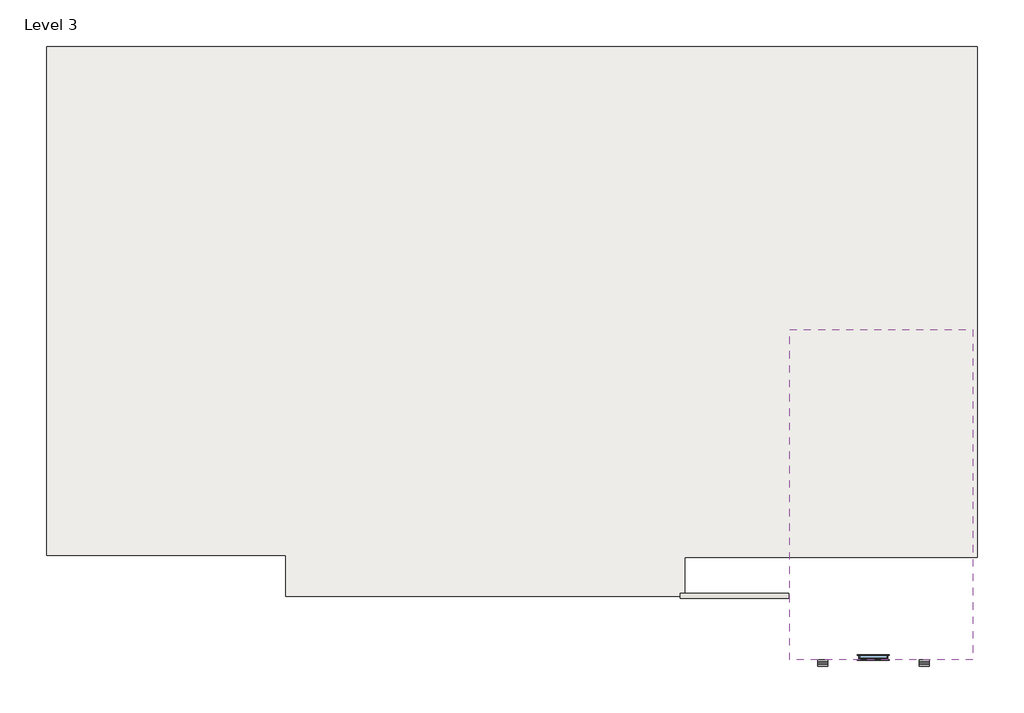
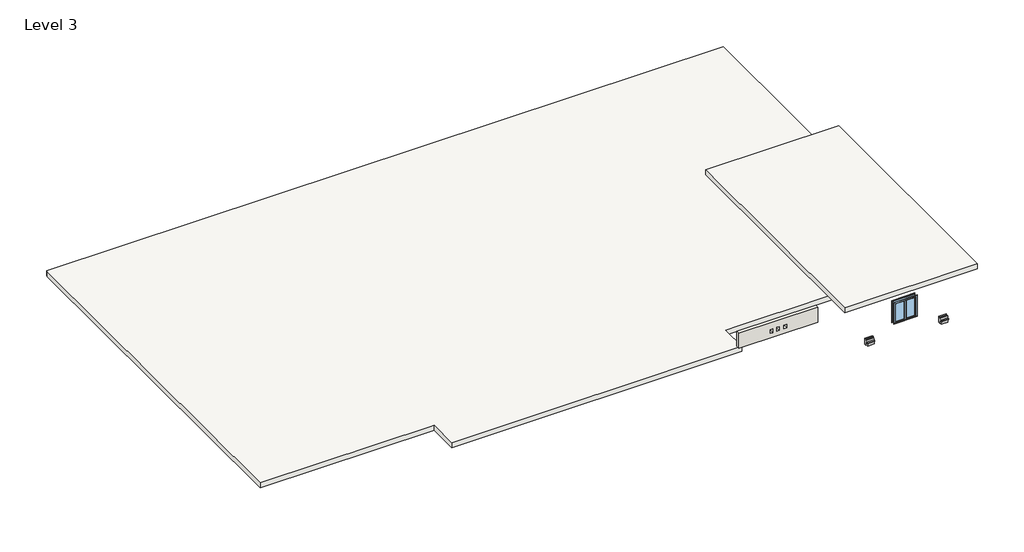
# One storey, incomplete: 2 light fixtures, 2 slabs, 1 wall, 1 window.
"""IFC4 building model written with IfcOpenShell, lengths in millimetres."""

from ifc_helpers import new_model, si_unit, frame, origin, place, context, project, spatial, polyline, outline, extrude, transform, mapped, element, save
from components import wall_pack_light_exterior_120v_ab60a804, window_0862ab64

model = new_model("IFC4")

# Units and contexts
model_context = context("Model", 3, world=origin())
ifc_project = project(units=[si_unit("LENGTHUNIT", "METRE", prefix="MILLI")], contexts=[model_context])

# Site, building, storey
site = spatial("IfcSite", under=ifc_project)
building = spatial("IfcBuilding", under=site)
storey = spatial("IfcBuildingStorey", under=building, Name="Level 3", Elevation=6400.8)

# Light fixtures
placement = place(None, origin())
wall_pack_light_exterior_120v_shape = wall_pack_light_exterior_120v_ab60a804(model_context)
element("IfcLightFixture", 1, ObjectType="Wall Pack Light - Exterior : 120V", at=placement, inside=storey, context=model_context, shape_type="MappedRepresentation", body=[
    mapped(wall_pack_light_exterior_120v_shape, transform((10185.0747398, -19224.6462052, 6389.2943487), x_axis=(1.0, 0.0, 0.0), y_axis=(0.0, 0.0, 1.0), z_axis=(0.0, -1.0, 0.0))),
])
element("IfcLightFixture", 2, ObjectType="Wall Pack Light - Exterior : 120V", at=placement, inside=storey, context=model_context, shape_type="MappedRepresentation", body=[
    mapped(wall_pack_light_exterior_120v_shape, transform((14452.2747398, -19224.6462052, 6224.0582374), x_axis=(1.0, 0.0, 0.0), y_axis=(0.0, 0.0, 1.0), z_axis=(0.0, -1.0, 0.0))),
])

# Slabs
element("IfcSlab", 3, ObjectType="Generic - 12\"", at=placement, inside=storey, context=model_context, shape_type="SweptSolid", body=[
    extrude(outline(polyline([(-22428.5252602, -14818.870124), (-22428.5252602, 6480.1537948), (-22428.5252602, 6567.929876), (16687.4747398, 6567.929876), (16687.4747398, -14920.470124), (4393.8747398, -14920.470124), (4393.8747398, -16555.9021378), (-12370.1252602, -16555.9021378), (-12370.1252602, -14818.870124), (-22428.5252602, -14818.870124)])), frame((0.0, 0.0, 6096.0), z_axis=(0.0, 0.0, 1.0), x_axis=(1.0, 0.0, 0.0)), (0.0, 0.0, 1.0), 304.8),
])
element("IfcSlab", 4, ObjectType="Generic - 12\"", at=placement, inside=storey, context=model_context, shape_type="SweptSolid", body=[
    extrude(outline(polyline([(16484.2747398, -5333.3996234), (16484.2747398, -19224.6462052), (8806.3760973, -19224.6462052), (8806.3760973, -5333.3996234), (16484.2747398, -5333.3996234)])), frame((0.0, 0.0, 8534.4), z_axis=(0.0, 0.0, 1.0), x_axis=(1.0, 0.0, 0.0)), (0.0, 0.0, 1.0), 304.8),
])

# Wall
element("IfcWall", 5, ObjectType="Generic - 8\"", at=placement, inside=storey, context=model_context, shape_type="SweptSolid", body=[
    extrude(outline(polyline([(6400.8, 4190.6747398), (6400.8, 8762.6747398), (7315.2, 8762.6747398), (7315.2, 4190.6747398), (6400.8, 4190.6747398)]), holes=[polyline([(6912.8521114, 6147.6437757), (6684.2521114, 6147.6437757), (6684.2521114, 5995.2437757), (6912.8521114, 5995.2437757), (6912.8521114, 6147.6437757)]), polyline([(6912.8521114, 6511.9432884), (6684.2521114, 6511.9432884), (6684.2521114, 6375.5920281), (6912.8521114, 6375.5920281), (6912.8521114, 6511.9432884)]), polyline([(6912.8521114, 6971.2317442), (6684.2521114, 6971.2317442), (6684.2521114, 6777.4694269), (6912.8521114, 6777.4694269), (6912.8521114, 6971.2317442)])]), frame((0.0, -16632.1021378, 0.0), z_axis=(0.0, 1.0, 0.0), x_axis=(0.0, 0.0, 1.0)), (0.0, 0.0, 1.0), 203.2),
])

# Window
window_shape = window_0862ab64(model_context)
element("IfcWindow", 6, ObjectType="Casement Dbl with Trim : 48\" x 48\"", at=placement, inside=storey, context=model_context, shape_type="MappedRepresentation", body=[
    mapped(window_shape, transform((12311.5760973, -19103.9962052, 5956.6910199), x_axis=(-1.0, 0.0, 0.0), y_axis=(0.0, -1.0, 0.0), z_axis=(0.0, 0.0, 1.0))),
])

save(model, "model.ifc")

# Revit data of these elements
# Type "Wall Pack Light - Exterior : 120V"
#   Photometric Web File = "WPE1MH.IES"
#   Wattage = 70 W
#   built-in parameter 1150110 = 1 (stored number, unit not read)
#   built-in parameter 1150109 = 1 (stored number, unit not read)
#   built-in parameter 1150113 = 1 (stored number, unit not read)
#   Tilt Angle = -90.00°
#   Lumens = 5499.9 lm
#   built-in parameter 1114217 = 1 (stored number, unit not read)
#   built-in parameter 1150115 = 1 (stored number, unit not read)
#   built-in parameter 1150105 = 437.668 (stored number, unit not read)
#   built-in parameter 1150112 = 1 (stored number, unit not read)
#   built-in parameter 1150114 = 1 (stored number, unit not read)
#   built-in parameter 1150107 = 4000 (stored number, unit not read)
#   built-in parameter 1150106 = 4.37668 (stored number, unit not read)
#   built-in parameter 1150104 = 7.29939 (stored number, unit not read)
#   Ballast Voltage = 120 V
#   Default Elevation = 9' - 0"
#   built-in parameter 1114218 = 1 (stored number, unit not read)
#   built-in parameter 1150133 = 10 (stored number, unit not read)
#   Apparent Load = 70 VA
#   built-in parameter 1150134 = 12
#   built-in parameter 1150137 = 1
#   Color Filter = 16777215
#   Ballast Number of Poles = 1
#   built-in parameter 1140040 [instance default] = 1
#   Wall Mount Material = Metal - Paint Finish - Dark Grey, Matte
#   Shade Material = Glass
#   Load Classification = Lighting - Exterior
#   Dimming Lamp Color Temperature Shift = (empty or 0)
# Type "Generic - 12\""
#   Assembly Code = "B1010"
#   Function = 0
#   Layers, outside or top first: 1' - 0" no material (function 1)
# Type "Generic - 8\""
#   Assembly Code = "B2010"
#   Layers, outside or top first: 0' - 8" no material (function 1)
# Type "Casement Dbl with Trim : 48\" x 48\""
#   Type Mark = "10"
#   Construction Type Id = "GSP4R"
#   Assembly Code = "B2020100"
#   Analytic Construction = "1/8 in Pilkington single glazing"
#   Visual Light Transmittance = 0.9
#   Solar Heat Gain Coefficient = 0.78
#   Heat Transfer Coefficient (U) = 0.6496 BTU/(h·ft²·°F)
#   Height = 4' - 0"
#   Default Sill Height = 3' - 0"
#   Trim Projection - Ext. = 0' - 0 1/2"
#   Trim Projection - Int. = 0' - 0 3/4"
#   Trim Width - Exterior = 0' - 3 1/2"
#   Trim Width - Interior = 0' - 3 1/2"
#   Width = 4' - 0"
#   Window Inset = 0' - 0 3/4"
#   Define Thermal Properties by = 1
#   Glass Pane Material = Glass
#   Sash Material = Glass
#   Trim Exterior Material = Glass, Clear Glazing
#   Trim Interior Material = Trim
#   Wall Closure = (empty or 0)
# Element 1 (IfcLightFixture, "Wall Pack Light - Exterior : 120V")
#   Mark = "1"
#   built-in parameter 1140040 = 1
#   Phase Created = New Construction
#   Materials on its faces: "Metal - Paint Finish - Dark Grey, Matte", "Glass"
# Element 2 (IfcLightFixture, "Wall Pack Light - Exterior : 120V")
#   Mark = "2"
#   built-in parameter 1140040 = 1
#   Phase Created = New Construction
#   Materials on its faces: "Metal - Paint Finish - Dark Grey, Matte", "Glass"
# Element 3 (IfcSlab, "Generic - 12\"")
#   built-in parameter 1001955 = -1.5708 (stored number, unit not read)
#   Height Offset From Level = 0' - 0"
#   Phase Created = New Construction
#   Materials on its faces: "Default Floor"
# Element 4 (IfcSlab, "Generic - 12\"")
#   Height Offset From Level = 8' - 0"
#   Phase Created = New Construction
#   Materials on its faces: "Default Floor"
# Element 5 (IfcWall, "Generic - 8\"")
#   Top Offset = 0' - 0"
#   Base Offset = 0' - 0"
#   Unconnected Height = 3' - 0"
#   wall height = 3' - 0"
#   Phase Created = New Construction
#   Base Constraint = Level 3
#   Materials on its faces: "Default Wall"
# Element 6 (IfcWindow, "Casement Dbl with Trim : 48\" x 48\"")
#   Mark = "3"
#   Phase Created = New Construction
#   Materials on its faces: "Glass", "Glass, Clear Glazing", "Trim"
# Materials
#   "Metal - Paint Finish - Dark Grey, Matte": class "Paint", colour RGB 98 98 98, transparency 0
#   "Glass": class "Glass", colour RGB 0 128 192, transparency 0.75, Description = "Soda Lime Glass", Cost = 0
#   "Glass, Clear Glazing": class "Glass", colour RGB 0 128 192, transparency 0.75, Description = "Clear glazing", Cost = 0
#   "Trim": class "Wood", colour RGB 224 178 126, transparency 0
#   "Default Floor": colour RGB 128 128 128, transparency 0
#   "Default Wall": colour RGB 128 128 128, transparency 0
